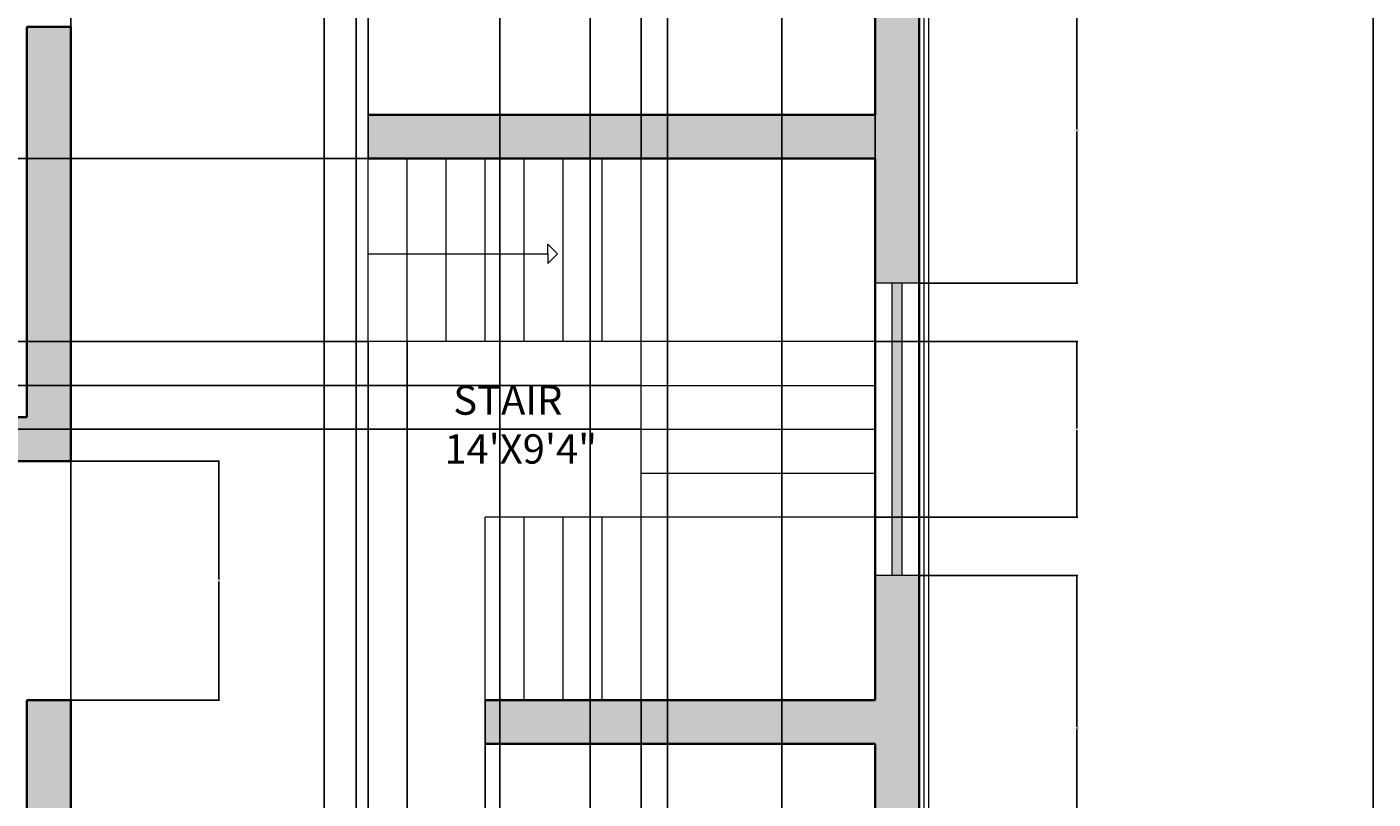
# Model space of a CAD drawing. Units: inches. Extents: x 311 to 815, y -527 to 136.
# Tile 14 of 21: x 539 to 815, y -368 to -210. Entities that reach past the tile are written whole.
import ezdxf

# ---------------------------------------------------------------- set-up
doc = ezdxf.new("R2010")
doc.units = ezdxf.units.IN
doc.header["$MEASUREMENT"] = 0
for name, color, linetype, lineweight in [('A-ANNO-DIMS', 1, 'Continuous', 18), ('A-ANNO-SYMB', 1, 'Continuous', 18), ('A-ANNO-TTLB', 1, 'Continuous', 25), ('A-AREA-IDEN', 8, 'Continuous', 18), ('A-FLOR-EDGE', 1, 'Continuous', 18), ('A-FLOR-STRS', 1, 'Continuous', 18), ('A-GLAZ-PATT', 5, 'Continuous', 13), ('A-WALL-PATT', 242, 'Continuous', 13), ('wall', 1, 'Continuous', 35), ('win', 5, 'Continuous', 18)]:
    doc.layers.add(name, color=color, linetype=linetype, lineweight=lineweight)
doc.styles.get("Standard").update_dxf_attribs({"font": 'arial.ttf'})
doc.dimstyles.get("Standard").update_dxf_attribs({"dimtxt": 0.18, "dimasz": 0.18, "dimexe": 0.18, "dimexo": 0.0625, "dimgap": 0.09, "dimtad": 0, "dimtih": 1, "dimtoh": 1, "dimdec": 1, "dimzin": 0, "dimdsep": 46, "dimlunit": 4, "dimtxsty": 'Standard', "dimcen": 0.09, "dimadec": 0, "dimazin": 0, "dimtfac": 1, "dimtdec": 1, "dimtofl": 0, "dimtmove": 0, "dimatfit": 3, "dimfxl": 1, "dimtolj": 1, "dimtzin": 0, "dimarcsym": 0})

# ---------------------------------------------------------------- blocks, each defined once
blk = doc.blocks.new('WIN-60IN')
for p, q in [((9, 60), (0, 60)), ((3.5, 0), (3.5, 60)), ((5.5, 0), (5.5, 60)), ((9, 0), (0, 0))]:
    blk.add_line(p, q)
blk = doc.blocks.new('*D25')
at = {"layer": 'A-ANNO-DIMS', "color": 0, "lineweight": -2, "transparency": 16777216}
for p, q in [((606.82, -473.07), (606.82, 54.4)), ((607, 54.22), (630.49, 54.22)), ((654.64, 54.22), (631.16, 54.22)), ((654.82, -473.07), (654.82, 54.4))]:
    blk.add_line(p, q, dxfattribs=at)
at = {"layer": 'A-ANNO-DIMS', "color": 0, "transparency": 16777216}
for points in [[(607, 54.25), (607, 54.19), (606.82, 54.22)], [(654.64, 54.25), (654.64, 54.19), (654.82, 54.22)]]:
    blk.add_solid(points, dxfattribs=at)
at = {"layer": 'Defpoints', "color": 0, "transparency": 16777216}
for p in [(654.82, 54.22), (606.82, -473.13), (654.82, -473.13)]:
    blk.add_point(p, dxfattribs=at)
at = {"layer": 'A-ANNO-DIMS', "color": 0, "transparency": 16777216, "insert": (630.82, 54.22), "char_height": 0.18, "attachment_point": 5}
blk.add_mtext('\\A1;4\'-0"', dxfattribs=at)
blk = doc.blocks.new('*D27')
at = {"layer": 'A-ANNO-DIMS', "color": 0, "lineweight": -2, "transparency": 16777216}
for p, q in [((548.32, -473.07), (548.32, 54.4)), ((548.5, 54.22), (576.96, 54.22)), ((606.64, 54.22), (578.19, 54.22)), ((606.82, -473.07), (606.82, 54.4))]:
    blk.add_line(p, q, dxfattribs=at)
at = {"layer": 'A-ANNO-DIMS', "color": 0, "transparency": 16777216}
for points in [[(548.5, 54.25), (548.5, 54.19), (548.32, 54.22)], [(606.64, 54.25), (606.64, 54.19), (606.82, 54.22)]]:
    blk.add_solid(points, dxfattribs=at)
at = {"layer": 'Defpoints', "color": 0, "transparency": 16777216}
for p in [(606.82, 54.22), (548.32, -473.13), (606.82, -473.13)]:
    blk.add_point(p, dxfattribs=at)
at = {"layer": 'A-ANNO-DIMS', "color": 0, "transparency": 16777216, "insert": (577.57, 54.22), "char_height": 0.18, "attachment_point": 5}
blk.add_mtext('\\A1;4\'-10 1/2"', dxfattribs=at)
blk = doc.blocks.new('*D28')
at = {"layer": 'A-ANNO-DIMS', "color": 0, "lineweight": -2, "transparency": 16777216}
for p, q in [((722.39, -322.63), (754.85, -322.63)), ((754.67, -322.81), (754.67, -353.69)), ((754.67, -384.95), (754.67, -354.06)), ((722.39, -385.13), (754.85, -385.13))]:
    blk.add_line(p, q, dxfattribs=at)
at = {"layer": 'A-ANNO-DIMS', "color": 0, "transparency": 16777216}
for points in [[(754.64, -322.81), (754.7, -322.81), (754.67, -322.63)], [(754.64, -384.95), (754.7, -384.95), (754.67, -385.13)]]:
    blk.add_solid(points, dxfattribs=at)
at = {"layer": 'Defpoints', "color": 0, "transparency": 16777216}
for p in [(722.32, -322.63), (722.32, -385.13), (754.67, -385.13)]:
    blk.add_point(p, dxfattribs=at)
at = {"layer": 'A-ANNO-DIMS', "color": 0, "transparency": 16777216, "insert": (754.67, -353.88), "char_height": 0.18, "attachment_point": 5}
blk.add_mtext('\\A1;5\'-2 1/2"', dxfattribs=at)
blk = doc.blocks.new('*D29')
at = {"layer": 'A-ANNO-DIMS', "color": 0, "lineweight": -2, "transparency": 16777216}
for p, q in [((722.39, -200.13), (754.85, -200.13)), ((754.67, -200.31), (754.67, -231.19)), ((754.67, -262.45), (754.67, -231.56)), ((722.39, -262.63), (754.85, -262.63))]:
    blk.add_line(p, q, dxfattribs=at)
at = {"layer": 'A-ANNO-DIMS', "color": 0, "transparency": 16777216}
for points in [[(754.64, -200.31), (754.7, -200.31), (754.67, -200.13)], [(754.64, -262.45), (754.7, -262.45), (754.67, -262.63)]]:
    blk.add_solid(points, dxfattribs=at)
at = {"layer": 'Defpoints', "color": 0, "transparency": 16777216}
for p in [(722.32, -200.13), (722.32, -262.63), (754.67, -262.63)]:
    blk.add_point(p, dxfattribs=at)
at = {"layer": 'A-ANNO-DIMS', "color": 0, "transparency": 16777216, "insert": (754.67, -231.38), "char_height": 0.18, "attachment_point": 5}
blk.add_mtext('\\A1;5\'-2 1/2"', dxfattribs=at)
blk = doc.blocks.new('*D31')
at = {"layer": 'A-ANNO-DIMS', "color": 0, "lineweight": -2, "transparency": 16777216}
for p, q in [((670.7, -191.61), (670.7, -526.66)), ((694.16, -191.61), (694.16, -526.66)), ((670.88, -526.48), (681.83, -526.48)), ((693.98, -526.48), (683.03, -526.48))]:
    blk.add_line(p, q, dxfattribs=at)
at = {"layer": 'A-ANNO-DIMS', "color": 0, "transparency": 16777216}
for points in [[(670.88, -526.45), (670.88, -526.51), (670.7, -526.48)], [(693.98, -526.45), (693.98, -526.51), (694.16, -526.48)]]:
    blk.add_solid(points, dxfattribs=at)
at = {"layer": 'Defpoints', "color": 0, "transparency": 16777216}
for p in [(670.7, -191.55), (694.16, -191.55), (694.16, -526.48)]:
    blk.add_point(p, dxfattribs=at)
at = {"layer": 'A-ANNO-DIMS', "color": 0, "transparency": 16777216, "insert": (682.43, -526.48), "char_height": 0.18, "attachment_point": 5}
blk.add_mtext('\\A1;1\'-11 1/2"', dxfattribs=at)
blk = doc.blocks.new('*D33')
at = {"layer": 'A-ANNO-DIMS', "color": 0, "lineweight": -2, "transparency": 16777216}
for p, q in [((609.26, -237.13), (377.79, -237.13)), ((377.97, -237.31), (377.97, -255.69)), ((377.97, -274.45), (377.97, -256.06)), ((609.26, -274.63), (377.79, -274.63))]:
    blk.add_line(p, q, dxfattribs=at)
at = {"layer": 'A-ANNO-DIMS', "color": 0, "transparency": 16777216}
for points in [[(377.94, -237.31), (378, -237.31), (377.97, -237.13)], [(377.94, -274.45), (378, -274.45), (377.97, -274.63)]]:
    blk.add_solid(points, dxfattribs=at)
at = {"layer": 'Defpoints', "color": 0, "transparency": 16777216}
for p in [(609.32, -237.13), (377.97, -274.63), (609.32, -274.63)]:
    blk.add_point(p, dxfattribs=at)
at = {"layer": 'A-ANNO-DIMS', "color": 0, "transparency": 16777216, "insert": (377.97, -255.88), "char_height": 0.18, "attachment_point": 5}
blk.add_mtext('\\A1;3\'-1 1/2"', dxfattribs=at)
blk = doc.blocks.new('*D34')
at = {"layer": 'A-ANNO-DIMS', "color": 0, "lineweight": -2, "transparency": 16777216}
for p, q in [((609.32, -274.69), (609.32, -526.66)), ((617.32, -274.69), (617.32, -526.66)), ((609.5, -526.48), (612.99, -526.48)), ((617.14, -526.48), (613.65, -526.48))]:
    blk.add_line(p, q, dxfattribs=at)
at = {"layer": 'A-ANNO-DIMS', "color": 0, "transparency": 16777216}
for points in [[(609.5, -526.45), (609.5, -526.51), (609.32, -526.48)], [(617.14, -526.45), (617.14, -526.51), (617.32, -526.48)]]:
    blk.add_solid(points, dxfattribs=at)
at = {"layer": 'Defpoints', "color": 0, "transparency": 16777216}
for p in [(609.32, -274.63), (617.32, -274.63), (617.32, -526.48)]:
    blk.add_point(p, dxfattribs=at)
at = {"layer": 'A-ANNO-DIMS', "color": 0, "transparency": 16777216, "insert": (613.32, -526.48), "char_height": 0.18, "attachment_point": 5}
blk.add_mtext('\\A1;0\'-8"', dxfattribs=at)
blk = doc.blocks.new('*D35')
at = {"layer": 'A-ANNO-DIMS', "color": 0, "lineweight": -2, "transparency": 16777216}
for p, q in [((665.32, -237.07), (665.32, 54.4)), ((665.5, 54.22), (688.99, 54.22)), ((713.14, 54.22), (689.66, 54.22)), ((713.32, -237.07), (713.32, 54.4))]:
    blk.add_line(p, q, dxfattribs=at)
at = {"layer": 'A-ANNO-DIMS', "color": 0, "transparency": 16777216}
for points in [[(665.5, 54.25), (665.5, 54.19), (665.32, 54.22)], [(713.14, 54.25), (713.14, 54.19), (713.32, 54.22)]]:
    blk.add_solid(points, dxfattribs=at)
at = {"layer": 'Defpoints', "color": 0, "transparency": 16777216}
for p in [(713.32, 54.22), (665.32, -237.13), (713.32, -237.13)]:
    blk.add_point(p, dxfattribs=at)
at = {"layer": 'A-ANNO-DIMS', "color": 0, "transparency": 16777216, "insert": (689.32, 54.22), "char_height": 0.18, "attachment_point": 5}
blk.add_mtext('\\A1;4\'-0"', dxfattribs=at)
blk = doc.blocks.new('*D36')
at = {"layer": 'A-ANNO-DIMS', "color": 0, "lineweight": -2, "transparency": 16777216}
for p, q in [((665.26, -283.63), (377.79, -283.63)), ((377.97, -283.81), (377.97, -287.95)), ((377.97, -292.45), (377.97, -288.31)), ((665.26, -292.63), (377.79, -292.63))]:
    blk.add_line(p, q, dxfattribs=at)
at = {"layer": 'A-ANNO-DIMS', "color": 0, "transparency": 16777216}
for points in [[(377.94, -283.81), (378, -283.81), (377.97, -283.63)], [(377.94, -292.45), (378, -292.45), (377.97, -292.63)]]:
    blk.add_solid(points, dxfattribs=at)
at = {"layer": 'Defpoints', "color": 0, "transparency": 16777216}
for p in [(665.32, -283.63), (377.97, -292.63), (665.32, -292.63)]:
    blk.add_point(p, dxfattribs=at)
at = {"layer": 'A-ANNO-DIMS', "color": 0, "transparency": 16777216, "insert": (377.97, -288.13), "char_height": 0.18, "attachment_point": 5}
blk.add_mtext('\\A1;0\'-9"', dxfattribs=at)
blk = doc.blocks.new('*D37')
at = {"layer": 'A-ANNO-DIMS', "color": 0, "lineweight": -2, "transparency": 16777216}
for p, q in [((633.32, -348.19), (633.32, -526.66)), ((665.32, -348.19), (665.32, -526.66)), ((633.5, -526.48), (648.99, -526.48)), ((665.14, -526.48), (649.65, -526.48))]:
    blk.add_line(p, q, dxfattribs=at)
at = {"layer": 'A-ANNO-DIMS', "color": 0, "transparency": 16777216}
for points in [[(633.5, -526.45), (633.5, -526.51), (633.32, -526.48)], [(665.14, -526.45), (665.14, -526.51), (665.32, -526.48)]]:
    blk.add_solid(points, dxfattribs=at)
at = {"layer": 'Defpoints', "color": 0, "transparency": 16777216}
for p in [(633.32, -348.13), (665.32, -348.13), (665.32, -526.48)]:
    blk.add_point(p, dxfattribs=at)
at = {"layer": 'A-ANNO-DIMS', "color": 0, "transparency": 16777216, "insert": (649.32, -526.48), "char_height": 0.18, "attachment_point": 5}
blk.add_mtext('\\A1;2\'-8"', dxfattribs=at)
blk = doc.blocks.new('*D38')
at = {"layer": 'A-ANNO-DIMS', "color": 0, "lineweight": -2, "transparency": 16777216}
for p, q in [((609.32, -237.07), (609.32, 54.4)), ((609.5, 54.22), (636.99, 54.22)), ((665.14, 54.22), (637.66, 54.22)), ((665.32, -237.07), (665.32, 54.4))]:
    blk.add_line(p, q, dxfattribs=at)
at = {"layer": 'A-ANNO-DIMS', "color": 0, "transparency": 16777216}
for points in [[(609.5, 54.25), (609.5, 54.19), (609.32, 54.22)], [(665.14, 54.25), (665.14, 54.19), (665.32, 54.22)]]:
    blk.add_solid(points, dxfattribs=at)
at = {"layer": 'Defpoints', "color": 0, "transparency": 16777216}
for p in [(665.32, 54.22), (609.32, -237.13), (665.32, -237.13)]:
    blk.add_point(p, dxfattribs=at)
at = {"layer": 'A-ANNO-DIMS', "color": 0, "transparency": 16777216, "insert": (637.32, 54.22), "char_height": 0.18, "attachment_point": 5}
blk.add_mtext('\\A1;4\'-8"', dxfattribs=at)
blk = doc.blocks.new('*D39')
at = {"layer": 'A-ANNO-DIMS', "color": 0, "lineweight": -2, "transparency": 16777216}
for p, q in [((713.39, -274.63), (754.85, -274.63)), ((754.67, -274.81), (754.67, -292.45)), ((754.67, -310.45), (754.67, -292.81)), ((713.39, -310.63), (754.85, -310.63))]:
    blk.add_line(p, q, dxfattribs=at)
at = {"layer": 'A-ANNO-DIMS', "color": 0, "transparency": 16777216}
for points in [[(754.64, -274.81), (754.7, -274.81), (754.67, -274.63)], [(754.64, -310.45), (754.7, -310.45), (754.67, -310.63)]]:
    blk.add_solid(points, dxfattribs=at)
at = {"layer": 'Defpoints', "color": 0, "transparency": 16777216}
for p in [(713.32, -274.63), (713.32, -310.63), (754.67, -310.63)]:
    blk.add_point(p, dxfattribs=at)
at = {"layer": 'A-ANNO-DIMS', "color": 0, "transparency": 16777216, "insert": (754.67, -292.63), "char_height": 0.18, "attachment_point": 5}
blk.add_mtext('\\A1;3\'-0"', dxfattribs=at)
blk = doc.blocks.new('*D49')
at = {"layer": 'A-ANNO-DIMS', "color": 0, "lineweight": -2, "transparency": 16777216}
for p, q in [((600.32, -112.19), (600.32, -526.66)), ((636.32, -112.19), (636.32, -526.66)), ((600.5, -526.48), (617.99, -526.48)), ((636.14, -526.48), (618.65, -526.48))]:
    blk.add_line(p, q, dxfattribs=at)
at = {"layer": 'A-ANNO-DIMS', "color": 0, "transparency": 16777216}
for points in [[(600.5, -526.45), (600.5, -526.51), (600.32, -526.48)], [(636.14, -526.45), (636.14, -526.51), (636.32, -526.48)]]:
    blk.add_solid(points, dxfattribs=at)
at = {"layer": 'Defpoints', "color": 0, "transparency": 16777216}
for p in [(600.32, -112.13), (636.32, -112.13), (636.32, -526.48)]:
    blk.add_point(p, dxfattribs=at)
at = {"layer": 'A-ANNO-DIMS', "color": 0, "transparency": 16777216, "insert": (618.32, -526.48), "char_height": 0.18, "attachment_point": 5}
blk.add_mtext('\\A1;3\'-0"', dxfattribs=at)
blk = doc.blocks.new('*D53')
at = {"layer": 'A-ANNO-DIMS', "color": 0, "lineweight": -2, "transparency": 16777216}
for p, q in [((548.39, -299.13), (578.85, -299.13)), ((578.67, -299.31), (578.67, -323.45)), ((578.67, -347.95), (578.67, -323.81)), ((548.39, -348.13), (578.85, -348.13))]:
    blk.add_line(p, q, dxfattribs=at)
at = {"layer": 'A-ANNO-DIMS', "color": 0, "transparency": 16777216}
for points in [[(578.64, -299.31), (578.7, -299.31), (578.67, -299.13)], [(578.64, -347.95), (578.7, -347.95), (578.67, -348.13)]]:
    blk.add_solid(points, dxfattribs=at)
at = {"layer": 'Defpoints', "color": 0, "transparency": 16777216}
for p in [(548.32, -299.13), (548.32, -348.13), (578.67, -348.13)]:
    blk.add_point(p, dxfattribs=at)
at = {"layer": 'A-ANNO-DIMS', "color": 0, "transparency": 16777216, "insert": (578.67, -323.63), "char_height": 0.18, "attachment_point": 5}
blk.add_mtext('\\A1;4\'-1"', dxfattribs=at)

msp = doc.modelspace()

# ---------------------------------------------------------------- hatches: boundary and pattern name
at = {"layer": 'A-GLAZ-PATT'}
h = msp.add_hatch(color=256, dxfattribs=at)
h.dxf.hatch_style = 1
h.paths.add_polyline_path([(415.82, -202.13), (413.82, -202.13), (413.82, -262.13), (415.82, -262.13)])
h.paths.add_polyline_path([(415.82, -390.84), (413.82, -390.84), (413.82, -450.84), (415.82, -450.84)])
h.paths.add_polyline_path([(415.82, -311.57), (413.82, -311.57), (413.82, -335.57), (415.82, -335.57)])
h.paths.add_polyline_path([(509.32, -476.63), (449.32, -476.63), (449.32, -478.63), (509.32, -478.63)])
h.paths.add_polyline_path([(606.82, -476.63), (582.82, -476.63), (582.82, -478.63), (606.82, -478.63)])
h.paths.add_polyline_path([(678.82, -476.63), (654.82, -476.63), (654.82, -478.63), (678.82, -478.63)])
h.paths.add_polyline_path([(718.82, -385.13), (716.82, -385.13), (716.82, -445.13), (718.82, -445.13)])
h.paths.add_polyline_path([(718.82, -262.63), (716.82, -262.63), (716.82, -322.63), (718.82, -322.63)])
h.paths.add_polyline_path([(718.82, -140.13), (716.82, -140.13), (716.82, -200.13), (718.82, -200.13)])
h.paths.add_polyline_path([(718.82, -18.13), (716.82, -18.13), (716.82, -42.13), (718.82, -42.13)])
h.paths.add_polyline_path([(686.82, 18.37), (626.82, 18.37), (626.82, 16.37), (686.82, 16.37)])
h.paths.add_polyline_path([(581.82, 18.37), (557.82, 18.37), (557.82, 16.37), (581.82, 16.37)])
h.paths.add_polyline_path([(509.32, 18.37), (449.32, 18.37), (449.32, 16.37), (509.32, 16.37)])
at = {"layer": 'A-WALL-PATT'}
h = msp.add_hatch(color=256, dxfattribs=at)
h.dxf.hatch_style = 1
h.paths.add_polyline_path([(557.82, 21.87), (509.32, 21.87), (509.32, 12.87), (539.32, 12.87), (539.32, -112.13), (548.32, -112.13), (548.32, -58.63), (557.82, -58.63), (557.82, -49.63), (548.32, -49.63), (548.32, 12.87), (557.82, 12.87)])
h.paths.add_polyline_path([(449.32, 21.87), (410.32, 21.87), (410.32, -15.13), (419.32, -15.13), (419.32, 12.87), (449.32, 12.87)])
h.paths.add_polyline_path([(626.82, 21.87), (581.82, 21.87), (581.82, 12.87), (591.32, 12.87), (591.32, -49.63), (581.82, -49.63), (581.82, -58.63), (591.32, -58.63), (591.32, -112.13), (600.32, -112.13), (600.32, 12.87), (626.82, 12.87)])
h.paths.add_polyline_path([(722.32, 21.87), (686.82, 21.87), (686.82, 12.87), (713.32, 12.87), (713.32, -18.13), (722.32, -18.13)])
h.paths.add_polyline_path([(722.32, -42.13), (713.32, -42.13), (713.32, -73.13), (722.32, -73.13)])
h.paths.add_polyline_path([(501.32, -103.13), (419.32, -103.13), (419.32, -75.13), (410.32, -75.13), (410.32, -126.63), (419.32, -126.63), (419.32, -112.13), (492.32, -112.13), (492.32, -143.13), (501.32, -143.13)])
h.paths.add_polyline_path([(548.32, -165.13), (419.32, -165.13), (419.32, -150.63), (410.32, -150.63), (410.32, -202.13), (419.32, -202.13), (419.32, -174.13), (548.32, -174.13)])
h.paths.add_polyline_path([(722.32, -103.13), (636.32, -103.13), (636.32, -112.13), (713.32, -112.13), (713.32, -140.13), (722.32, -140.13)])
h.paths.add_polyline_path([(548.32, -210.13), (539.32, -210.13), (539.32, -290.13), (419.32, -290.13), (419.32, -262.13), (410.32, -262.13), (410.32, -311.57), (419.32, -311.57), (419.32, -299.13), (469.32, -299.13), (469.32, -348.13), (443.32, -348.13), (443.32, -357.13), (478.32, -357.13), (478.32, -299.13), (548.32, -299.13)])
h.paths.add_polyline_path([(722.32, -200.13), (713.32, -200.13), (713.32, -228.13), (609.32, -228.13), (609.32, -237.13), (713.32, -237.13), (713.32, -262.63), (722.32, -262.63)])
h.paths.add_polyline_path([(722.32, -322.63), (713.32, -322.63), (713.32, -348.13), (633.32, -348.13), (633.32, -357.13), (713.32, -357.13), (713.32, -385.13), (722.32, -385.13)])
h.paths.add_polyline_path([(419.32, -335.57), (410.32, -335.57), (410.32, -390.84), (419.32, -390.84)])
h.paths.add_polyline_path([(419.32, -450.84), (410.32, -450.84), (410.32, -482.13), (449.32, -482.13), (449.32, -473.13), (419.32, -473.13)])
h.paths.add_polyline_path([(582.82, -473.13), (548.32, -473.13), (548.32, -348.13), (539.32, -348.13), (539.32, -473.13), (509.32, -473.13), (509.32, -482.13), (582.82, -482.13)])
h.paths.add_polyline_path([(722.32, -445.13), (713.32, -445.13), (713.32, -473.13), (678.82, -473.13), (678.82, -482.13), (722.32, -482.13)])

# ---------------------------------------------------------------- linework, layer by layer
at = {"layer": 'A-ANNO-SYMB'}
for p, q in [((609.32, -256.65), (646.15, -256.65)), ((646.15, -256.65), (646.15, -254.65)), ((648.15, -256.65), (646.15, -254.65)), ((646.15, -256.65), (646.15, -258.65)), ((648.15, -256.65), (646.15, -258.65))]:
    msp.add_line(p, q, dxfattribs=at)
at = {"layer": 'A-ANNO-TTLB'}
msp.add_lwpolyline([(310.67, 136.01), (815.43, 136.01), (815.43, -506.97), (310.67, -506.97)], close=True, dxfattribs=at)
at = {"layer": 'A-FLOR-EDGE'}
for p, q in [((723.32, -483.13), (723.32, 22.87)), ((724.32, -484.13), (724.32, 23.87))]:
    msp.add_line(p, q, dxfattribs=at)
at = {"layer": 'A-FLOR-STRS'}
for p, q in [((609.32, -274.63), (609.32, -228.13)), ((617.32, -274.63), (617.32, -237.13)), ((625.32, -274.63), (625.32, -237.13)), ((633.32, -274.63), (633.32, -237.13)), ((641.32, -274.63), (641.32, -237.13)), ((649.32, -274.63), (649.32, -237.13)), ((657.32, -274.63), (657.32, -237.13)), ((665.32, -348.13), (665.32, -237.13)), ((713.32, -274.63), (609.32, -274.63)), ((665.32, -283.63), (713.32, -283.63)), ((665.32, -292.63), (713.32, -292.63)), ((665.32, -301.63), (713.32, -301.63)), ((713.32, -310.63), (633.32, -310.63)), ((633.32, -357.13), (633.32, -310.63)), ((641.32, -348.13), (641.32, -310.63)), ((649.32, -348.13), (649.32, -310.63)), ((657.32, -348.13), (657.32, -310.63))]:
    msp.add_line(p, q, dxfattribs=at)
at = {"layer": 'wall'}
for p, q in [((722.32, -482.13), (722.32, -103.13)), ((713.32, -228.13), (713.32, -112.13)), ((548.32, -210.13), (539.32, -210.13)), ((539.32, -290.13), (539.32, -210.13)), ((548.32, -299.13), (548.32, -210.13)), ((713.32, -228.13), (609.32, -228.13)), ((713.32, -237.13), (609.32, -237.13)), ((713.32, -348.13), (713.32, -237.13)), ((539.32, -290.13), (419.32, -290.13)), ((548.32, -299.13), (478.32, -299.13)), ((539.32, -473.13), (539.32, -348.13)), ((539.32, -348.13), (548.32, -348.13)), ((539.32, -348.13), (548.32, -348.13)), ((548.32, -473.13), (548.32, -348.13)), ((633.32, -348.13), (713.32, -348.13)), ((633.32, -357.13), (713.32, -357.13)), ((713.32, -473.13), (713.32, -357.13))]:
    msp.add_line(p, q, dxfattribs=at)

# ---------------------------------------------------------------- block references
at = {"layer": 'win'}
msp.add_blockref('WIN-60IN', (713.32, -322.63), dxfattribs=at)

# ---------------------------------------------------------------- texts
at = {"layer": 'A-AREA-IDEN', "insert": (624.94, -283.63), "char_height": 6.0073, "attachment_point": 1}
msp.add_mtext_dynamic_manual_height_columns(' STAIR      14\'X9\'4"', width=29.2408, gutter_width=1, heights=[0], dxfattribs=at)

# ---------------------------------------------------------------- dimensions: what is measured, and where the dimension line sits
at = {"layer": 'A-ANNO-DIMS'}
for base, p1, p2, picture, middle in [((606.82, 54.22), (548.32, -473.13), (606.82, -473.13), '*D27', (577.57, 54.22)), ((654.82, 54.22), (606.82, -473.13), (654.82, -473.13), '*D25', (630.82, 54.22)), ((665.32, 54.22), (609.32, -237.13), (665.32, -237.13), '*D38', (637.32, 54.22)), ((713.32, 54.22), (665.32, -237.13), (713.32, -237.13), '*D35', (689.32, 54.22)), ((636.32, -526.48), (600.32, -112.13), (636.32, -112.13), '*D49', (618.32, -526.48)), ((694.16, -526.48), (670.7, -191.55), (694.16, -191.55), '*D31', (682.43, -526.48)), ((617.32, -526.48), (609.32, -274.63), (617.32, -274.63), '*D34', (613.32, -526.48)), ((665.32, -526.48), (633.32, -348.13), (665.32, -348.13), '*D37', (649.32, -526.48))]:
    dim = msp.add_linear_dim(base=base, p1=p1, p2=p2, dimstyle='Standard', override={"dimdec": 1, "dimlfac": 1, "dimrnd": 0, "dimzin": 1, "dimdsep": 46, "dimlunit": 4, "dimfrac": 2}, dxfattribs=at)
    dim.commit()
    dim.dimension.update_dxf_attribs({"geometry": picture, "text_midpoint": middle})
for base, p1, p2, angle, picture, middle in [((754.67, -262.63), (722.32, -200.13), (722.32, -262.63), 90, '*D29', (754.67, -231.38)), ((377.97, -274.63), (609.32, -237.13), (609.32, -274.63), 90, '*D33', (377.97, -255.88)), ((754.67, -310.63), (713.32, -274.63), (713.32, -310.63), 90, '*D39', (754.67, -292.63)), ((377.97, -292.63), (665.32, -283.63), (665.32, -292.63), 90, '*D36', (377.97, -288.13)), ((578.67, -348.13), (548.32, -299.13), (548.32, -348.13), 270, '*D53', (578.67, -323.63)), ((754.67, -385.13), (722.32, -322.63), (722.32, -385.13), 90, '*D28', (754.67, -353.88))]:
    dim = msp.add_linear_dim(base=base, p1=p1, p2=p2, angle=angle, dimstyle='Standard', override={"dimdec": 1, "dimlfac": 1, "dimrnd": 0, "dimzin": 1, "dimdsep": 46, "dimlunit": 4, "dimfrac": 2}, dxfattribs=at)
    dim.commit()
    dim.dimension.update_dxf_attribs({"geometry": picture, "text_midpoint": middle})

doc.saveas('drawing.dxf')
